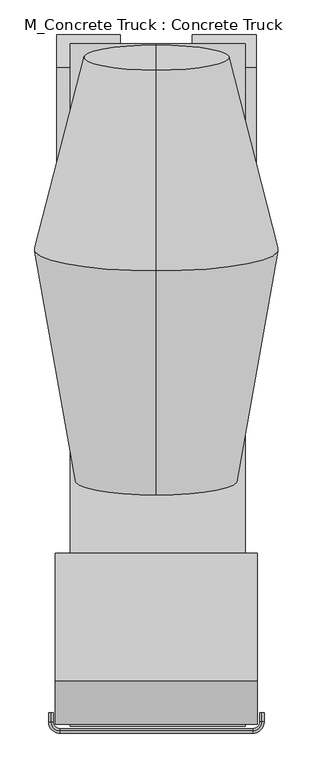
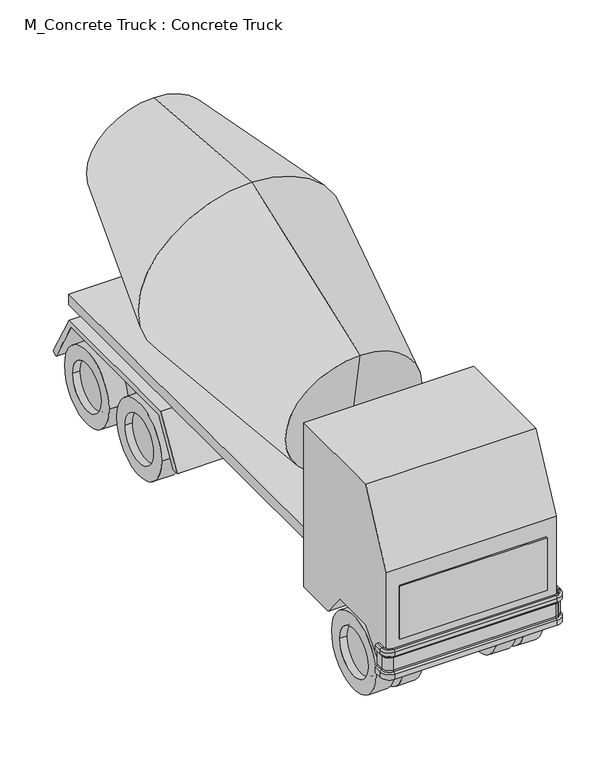
"""IFC4 building model written with IfcOpenShell, lengths in millimetres: geographic element geometry, M_Concrete Truck : Concrete Truck."""

from ifc_helpers import new_model, si_unit, point, frame, frame_2d, origin, place, context, project, spatial, polyline, circle_curve, ellipse_curve, trimmed, segment, composite_curve, outline, extrude, source, transform, mapped, element, save
from ifc_brep_helpers import plane_surface, cylinder_surface, revolved_surface, advanced_brep


def m_concrete_truck_concrete_truck_8dc9909d(model_context):
    return source(origin(), model_context, "Body", "SolidModel", [
        extrude(outline(polyline([(362.4384615, 3777.7615385), (362.4384615, -1683.2384615), (725.7603556, -1683.2384615), (725.7603556, -3004.0384615), (-798.2396444, -3004.0384615), (-798.2396444, -1683.2384615), (-450.3615385, -1683.2384615), (-450.3615385, 3777.7615385), (362.4384615, 3777.7615385)])), frame((0.0, 0.0, 711.2), z_axis=(0.0, 0.0, 1.0), x_axis=(1.0, 0.0, 0.0)), (0.0, 0.0, 1.0), 508.0),
        extrude(outline(composite_curve([segment(trimmed(circle_curve(frame_2d((3091.9615385, 514.35)), 520.7), [point((3612.6615385, 514.35))], [point((2571.2615385, 514.35))], False, "CARTESIAN"), True, "CONTINUOUS"), segment(trimmed(circle_curve(frame_2d((3091.9615385, 514.35)), 520.7), [point((2571.2615385, 514.35))], [point((3612.6615385, 514.35))], False, "CARTESIAN"), True, "CONTINUOUS")], self_intersect=False), holes=[composite_curve([segment(trimmed(circle_curve(frame_2d((3091.9615385, 514.35)), 330.2), [point((3422.1615385, 514.35))], [point((2761.7615385, 514.35))], True, "CARTESIAN"), True, "CONTINUOUS"), segment(trimmed(circle_curve(frame_2d((3091.9615385, 514.35)), 330.2), [point((2761.7615385, 514.35))], [point((3422.1615385, 514.35))], True, "CARTESIAN"), True, "CONTINUOUS")], self_intersect=False)]), frame((829.1634615, 0.0, 0.0), z_axis=(1.0, 0.0, 0.0), x_axis=(0.0, 1.0, 0.0)), (0.0, 0.0, 1.0), 254.0),
        extrude(outline(composite_curve([segment(trimmed(circle_curve(frame_2d((-3131.0384615, 514.35)), 520.7), [point((-2610.3384615, 514.35))], [point((-3651.7384615, 514.35))], False, "CARTESIAN"), True, "CONTINUOUS"), segment(trimmed(circle_curve(frame_2d((-3131.0384615, 514.35)), 520.7), [point((-3651.7384615, 514.35))], [point((-2610.3384615, 514.35))], False, "CARTESIAN"), True, "CONTINUOUS")], self_intersect=False), holes=[composite_curve([segment(trimmed(circle_curve(frame_2d((-3131.0384615, 514.35)), 330.2), [point((-2800.8384615, 514.35))], [point((-3461.2384615, 514.35))], True, "CARTESIAN"), True, "CONTINUOUS"), segment(trimmed(circle_curve(frame_2d((-3131.0384615, 514.35)), 330.2), [point((-3461.2384615, 514.35))], [point((-2800.8384615, 514.35))], True, "CARTESIAN"), True, "CONTINUOUS")], self_intersect=False)]), frame((829.1634615, 0.0, 0.0), z_axis=(1.0, 0.0, 0.0), x_axis=(0.0, 1.0, 0.0)), (0.0, 0.0, 1.0), 254.0),
        extrude(outline(composite_curve([segment(trimmed(circle_curve(frame_2d((1872.7615385, 514.35)), 520.7), [point((2393.4615385, 514.35))], [point((1352.0615385, 514.35))], False, "CARTESIAN"), True, "CONTINUOUS"), segment(trimmed(circle_curve(frame_2d((1872.7615385, 514.35)), 520.7), [point((1352.0615385, 514.35))], [point((2393.4615385, 514.35))], False, "CARTESIAN"), True, "CONTINUOUS")], self_intersect=False), holes=[composite_curve([segment(trimmed(circle_curve(frame_2d((1872.7615385, 514.35)), 330.2), [point((2202.9615385, 514.35))], [point((1542.5615385, 514.35))], True, "CARTESIAN"), True, "CONTINUOUS"), segment(trimmed(circle_curve(frame_2d((1872.7615385, 514.35)), 330.2), [point((1542.5615385, 514.35))], [point((2202.9615385, 514.35))], True, "CARTESIAN"), True, "CONTINUOUS")], self_intersect=False)]), frame((829.1634615, 0.0, 0.0), z_axis=(1.0, 0.0, 0.0), x_axis=(0.0, 1.0, 0.0)), (0.0, 0.0, 1.0), 254.0),
        advanced_brep(
        [(-1212.3615385, -3791.4384615, 661.0144121), (-1263.1615385, -3791.4384615, 661.0144121), (-1263.1615385, -3791.4384615, 734.1328754), (-1243.6602579, -3791.4384615, 753.634156), (-1236.2207701, -3791.4384615, 771.5946682), (-1236.2207701, -3791.4384615, 953.7526192), (-1243.6602579, -3791.4384615, 971.7131315), (-1263.1615385, -3791.4384615, 991.2144121), (-1263.1615385, -3791.4384615, 1042.0144121), (-1237.7615385, -3791.4384615, 1067.4144121), (-1212.3615385, -3791.4384615, 1067.4144121), (-1212.3615385, -3893.0384615, 661.0144121), (-1263.1615385, -3893.0384615, 661.0144121), (-1263.1615385, -3893.0384615, 734.1328754), (-1243.6602579, -3893.0384615, 753.634156), (-1236.2207701, -3893.0384615, 771.5946682), (-1236.2207701, -3893.0384615, 953.7526192), (-1243.6602579, -3893.0384615, 971.7131315), (-1263.1615385, -3893.0384615, 991.2144121), (-1263.1615385, -3893.0384615, 1042.0144121), (-1237.7615385, -3893.0384615, 1067.4144121), (-1212.3615385, -3893.0384615, 1067.4144121), (-1136.1615385, -4020.0384615, 661.0144121), (-1136.1615385, -3969.2384615, 661.0144121), (-1136.1615385, -4020.0384615, 734.1328754), (-1136.1615385, -4000.5371809, 753.634156), (-1136.1615385, -3993.0976932, 771.5946682), (-1136.1615385, -3993.0976932, 953.7526192), (-1136.1615385, -4000.5371809, 971.7131315), (-1136.1615385, -4020.0384615, 991.2144121), (-1136.1615385, -4020.0384615, 1042.0144121), (-1136.1615385, -3994.6384615, 1067.4144121), (-1136.1615385, -3969.2384615, 1067.4144121), (1048.2384615, -3969.2384615, 661.0144121), (1048.2384615, -4020.0384615, 661.0144121), (1048.2384615, -4020.0384615, 734.1328754), (1048.2384615, -4000.5371809, 753.634156), (1048.2384615, -3993.0976932, 771.5946682), (1048.2384615, -3993.0976932, 953.7526192), (1048.2384615, -4000.5371809, 971.7131315), (1048.2384615, -4020.0384615, 991.2144121), (1048.2384615, -4020.0384615, 1042.0144121), (1048.2384615, -3994.6384615, 1067.4144121), (1048.2384615, -3969.2384615, 1067.4144121), (1175.2384615, -3893.0384615, 661.0144121), (1124.4384615, -3893.0384615, 661.0144121), (1175.2384615, -3893.0384615, 734.1328754), (1155.7371809, -3893.0384615, 753.634156), (1148.2976932, -3893.0384615, 771.5946682), (1148.2976932, -3893.0384615, 953.7526192), (1155.7371809, -3893.0384615, 971.7131315), (1175.2384615, -3893.0384615, 991.2144121), (1175.2384615, -3893.0384615, 1042.0144121), (1149.8384615, -3893.0384615, 1067.4144121), (1124.4384615, -3893.0384615, 1067.4144121), (1124.4384615, -3791.4384615, 661.0144121), (1124.4384615, -3791.4384615, 1067.4144121), (1149.8384615, -3791.4384615, 1067.4144121), (1175.2384615, -3791.4384615, 1042.0144121), (1175.2384615, -3791.4384615, 991.2144121), (1155.7371809, -3791.4384615, 971.7131315), (1148.2976932, -3791.4384615, 953.7526192), (1148.2976932, -3791.4384615, 771.5946682), (1155.7371809, -3791.4384615, 753.634156), (1175.2384615, -3791.4384615, 734.1328754), (1175.2384615, -3791.4384615, 661.0144121)],
        [
            (0, 1),
            (1, 2),
            (2, 3),
            (3, 4, circle_curve(frame((-1261.6207701, -3791.4384615, 771.5946682), z_axis=(0.0, -1.0, 0.0), x_axis=(1.0, 0.0, 0.0)), 25.4)),
            (4, 5),
            (5, 6, circle_curve(frame((-1261.6207701, -3791.4384615, 953.7526192), z_axis=(0.0, -1.0, 0.0), x_axis=(1.0, 0.0, 0.0)), 25.4)),
            (6, 7),
            (7, 8),
            (8, 9, circle_curve(frame((-1237.7615385, -3791.4384615, 1042.0144121), z_axis=(0.0, 1.0, 0.0), x_axis=(1.0, 0.0, 0.0)), 25.4)),
            (9, 10),
            (10, 0),
            (0, 11),
            (11, 12),
            (12, 1),
            (12, 13),
            (13, 2),
            (13, 14),
            (14, 3),
            (14, 15, circle_curve(frame((-1261.6207701, -3893.0384615, 771.5946682), z_axis=(0.0, -1.0, 0.0), x_axis=(1.0, 0.0, 0.0)), 25.4)),
            (15, 4),
            (15, 16),
            (16, 5),
            (16, 17, circle_curve(frame((-1261.6207701, -3893.0384615, 953.7526192), z_axis=(0.0, -1.0, 0.0), x_axis=(1.0, 0.0, 0.0)), 25.4)),
            (17, 6),
            (17, 18),
            (18, 7),
            (18, 19),
            (19, 8),
            (19, 20, circle_curve(frame((-1237.7615385, -3893.0384615, 1042.0144121), z_axis=(0.0, 1.0, 0.0), x_axis=(1.0, 0.0, 0.0)), 25.4)),
            (20, 9),
            (20, 21),
            (21, 10),
            (21, 11),
            (22, 12, circle_curve(frame((-1136.1615385, -3893.0384615, 661.0144121), z_axis=(0.0, 0.0, -1.0), x_axis=(-1.0, 0.0, 0.0)), 127.0)),
            (11, 23, circle_curve(frame((-1136.1615385, -3893.0384615, 661.0144121), z_axis=(0.0, 0.0, 1.0), x_axis=(-1.0, 0.0, 0.0)), 76.2)),
            (23, 22),
            (24, 13, circle_curve(frame((-1136.1615385, -3893.0384615, 734.1328754), z_axis=(0.0, 0.0, -1.0), x_axis=(-1.0, 0.0, 0.0)), 127.0)),
            (22, 24),
            (25, 14, circle_curve(frame((-1136.1615385, -3893.0384615, 753.634156), z_axis=(0.0, 0.0, -1.0), x_axis=(-1.0, 0.0, 0.0)), 107.4987194)),
            (24, 25),
            (26, 15, circle_curve(frame((-1136.1615385, -3893.0384615, 771.5946682), z_axis=(0.0, 0.0, -1.0), x_axis=(-1.0, 0.0, 0.0)), 100.0592316)),
            (25, 26, circle_curve(frame((-1136.1615385, -4018.4976932, 771.5946682), z_axis=(1.0, 0.0, 0.0), x_axis=(0.0, 1.0, 0.0)), 25.4)),
            (27, 16, circle_curve(frame((-1136.1615385, -3893.0384615, 953.7526192), z_axis=(0.0, 0.0, -1.0), x_axis=(-1.0, 0.0, 0.0)), 100.0592316)),
            (26, 27),
            (28, 17, circle_curve(frame((-1136.1615385, -3893.0384615, 971.7131315), z_axis=(0.0, 0.0, -1.0), x_axis=(-1.0, 0.0, 0.0)), 107.4987194)),
            (27, 28, circle_curve(frame((-1136.1615385, -4018.4976932, 953.7526192), z_axis=(1.0, 0.0, 0.0), x_axis=(0.0, 1.0, 0.0)), 25.4)),
            (29, 18, circle_curve(frame((-1136.1615385, -3893.0384615, 991.2144121), z_axis=(0.0, 0.0, -1.0), x_axis=(-1.0, 0.0, 0.0)), 127.0)),
            (28, 29),
            (30, 19, circle_curve(frame((-1136.1615385, -3893.0384615, 1042.0144121), z_axis=(0.0, 0.0, -1.0), x_axis=(-1.0, 0.0, 0.0)), 127.0)),
            (29, 30),
            (31, 20, circle_curve(frame((-1136.1615385, -3893.0384615, 1067.4144121), z_axis=(0.0, 0.0, -1.0), x_axis=(-1.0, 0.0, 0.0)), 101.6)),
            (30, 31, circle_curve(frame((-1136.1615385, -3994.6384615, 1042.0144121), z_axis=(-1.0, 0.0, 0.0), x_axis=(0.0, 1.0, 0.0)), 25.4)),
            (32, 21, circle_curve(frame((-1136.1615385, -3893.0384615, 1067.4144121), z_axis=(0.0, 0.0, -1.0), x_axis=(-1.0, 0.0, 0.0)), 76.2)),
            (31, 32),
            (32, 23),
            (23, 33),
            (33, 34),
            (34, 22),
            (34, 35),
            (35, 24),
            (35, 36),
            (36, 25),
            (36, 37, circle_curve(frame((1048.2384615, -4018.4976932, 771.5946682), z_axis=(1.0, 0.0, 0.0), x_axis=(0.0, 1.0, 0.0)), 25.4)),
            (37, 26),
            (37, 38),
            (38, 27),
            (38, 39, circle_curve(frame((1048.2384615, -4018.4976932, 953.7526192), z_axis=(1.0, 0.0, 0.0), x_axis=(0.0, 1.0, 0.0)), 25.4)),
            (39, 28),
            (39, 40),
            (40, 29),
            (40, 41),
            (41, 30),
            (41, 42, circle_curve(frame((1048.2384615, -3994.6384615, 1042.0144121), z_axis=(-1.0, 0.0, 0.0), x_axis=(0.0, 1.0, 0.0)), 25.4)),
            (42, 31),
            (42, 43),
            (43, 32),
            (43, 33),
            (44, 34, circle_curve(frame((1048.2384615, -3893.0384615, 661.0144121), z_axis=(0.0, 0.0, -1.0), x_axis=(0.0, -1.0, 0.0)), 127.0)),
            (33, 45, circle_curve(frame((1048.2384615, -3893.0384615, 661.0144121), z_axis=(0.0, 0.0, 1.0), x_axis=(0.0, -1.0, 0.0)), 76.2)),
            (45, 44),
            (46, 35, circle_curve(frame((1048.2384615, -3893.0384615, 734.1328754), z_axis=(0.0, 0.0, -1.0), x_axis=(0.0, -1.0, 0.0)), 127.0)),
            (44, 46),
            (47, 36, circle_curve(frame((1048.2384615, -3893.0384615, 753.634156), z_axis=(0.0, 0.0, -1.0), x_axis=(0.0, -1.0, 0.0)), 107.4987194)),
            (46, 47),
            (48, 37, circle_curve(frame((1048.2384615, -3893.0384615, 771.5946682), z_axis=(0.0, 0.0, -1.0), x_axis=(0.0, -1.0, 0.0)), 100.0592316)),
            (47, 48, circle_curve(frame((1173.6976932, -3893.0384615, 771.5946682), z_axis=(0.0, 1.0, 0.0), x_axis=(-1.0, 0.0, 0.0)), 25.4)),
            (49, 38, circle_curve(frame((1048.2384615, -3893.0384615, 953.7526192), z_axis=(0.0, 0.0, -1.0), x_axis=(0.0, -1.0, 0.0)), 100.0592316)),
            (48, 49),
            (50, 39, circle_curve(frame((1048.2384615, -3893.0384615, 971.7131315), z_axis=(0.0, 0.0, -1.0), x_axis=(0.0, -1.0, 0.0)), 107.4987194)),
            (49, 50, circle_curve(frame((1173.6976932, -3893.0384615, 953.7526192), z_axis=(0.0, 1.0, 0.0), x_axis=(-1.0, 0.0, 0.0)), 25.4)),
            (51, 40, circle_curve(frame((1048.2384615, -3893.0384615, 991.2144121), z_axis=(0.0, 0.0, -1.0), x_axis=(0.0, -1.0, 0.0)), 127.0)),
            (50, 51),
            (52, 41, circle_curve(frame((1048.2384615, -3893.0384615, 1042.0144121), z_axis=(0.0, 0.0, -1.0), x_axis=(0.0, -1.0, 0.0)), 127.0)),
            (51, 52),
            (53, 42, circle_curve(frame((1048.2384615, -3893.0384615, 1067.4144121), z_axis=(0.0, 0.0, -1.0), x_axis=(0.0, -1.0, 0.0)), 101.6)),
            (52, 53, circle_curve(frame((1149.8384615, -3893.0384615, 1042.0144121), z_axis=(0.0, -1.0, 0.0), x_axis=(-1.0, 0.0, 0.0)), 25.4)),
            (54, 43, circle_curve(frame((1048.2384615, -3893.0384615, 1067.4144121), z_axis=(0.0, 0.0, -1.0), x_axis=(0.0, -1.0, 0.0)), 76.2)),
            (53, 54),
            (54, 45),
            (55, 56),
            (56, 57),
            (57, 58, circle_curve(frame((1149.8384615, -3791.4384615, 1042.0144121), z_axis=(0.0, 1.0, 0.0), x_axis=(-1.0, 0.0, 0.0)), 25.4)),
            (58, 59),
            (59, 60),
            (60, 61, circle_curve(frame((1173.6976932, -3791.4384615, 953.7526192), z_axis=(0.0, -1.0, 0.0), x_axis=(-1.0, 0.0, 0.0)), 25.4)),
            (61, 62),
            (62, 63, circle_curve(frame((1173.6976932, -3791.4384615, 771.5946682), z_axis=(0.0, -1.0, 0.0), x_axis=(-1.0, 0.0, 0.0)), 25.4)),
            (63, 64),
            (64, 65),
            (65, 55),
            (45, 55),
            (65, 44),
            (64, 46),
            (63, 47),
            (62, 48),
            (61, 49),
            (60, 50),
            (59, 51),
            (58, 52),
            (57, 53),
            (56, 54),
        ],
        [
            plane_surface(frame((-2331.7840944, -3791.4384615, 0.0), z_axis=(0.0, 1.0, 0.0), x_axis=(0.0, 0.0, -1.0))),
            plane_surface(frame((-1212.3615385, -3791.4384615, 661.0144121), z_axis=(0.0, 0.0, -1.0), x_axis=(0.0, -1.0, 0.0))),
            plane_surface(frame((-1263.1615385, -3791.4384615, 661.0144121), z_axis=(-1.0, 0.0, 0.0), x_axis=(0.0, -1.0, 0.0))),
            plane_surface(frame((-1263.1615385, -3791.4384615, 734.1328754), z_axis=(-0.7071067811866113, 0.0, 0.7071067811864837), x_axis=(0.0, -1.0, 0.0))),
            revolved_surface(polyline([(-1236.2207701, -3893.0384615, 771.5946682), (-1236.2207701, -3791.4384615, 771.5946682)]), (-1261.6207701, -3791.4384615, 771.5946682), (0.0, -1.0, 0.0)),
            plane_surface(frame((-1236.2207701, -3791.4384615, 771.5946682), z_axis=(-1.0, 0.0, 0.0), x_axis=(0.0, -1.0, 0.0))),
            revolved_surface(polyline([(-1236.2207701, -3893.0384615, 953.7526192), (-1236.2207701, -3791.4384615, 953.7526192)]), (-1261.6207701, -3791.4384615, 953.7526192), (0.0, -1.0, 0.0)),
            plane_surface(frame((-1243.6602579, -3791.4384615, 971.7131315), z_axis=(-0.7071067811866555, 0.0, -0.7071067811864395), x_axis=(0.0, -1.0, 0.0))),
            plane_surface(frame((-1263.1615385, -3791.4384615, 991.2144121), z_axis=(-1.0, 0.0, 0.0), x_axis=(0.0, -1.0, 0.0))),
            cylinder_surface(frame((-1237.7615385, -3791.4384615, 1042.0144121), z_axis=(0.0, 1.0, 0.0), x_axis=(1.0, 0.0, 0.0)), 25.4),
            plane_surface(frame((-1237.7615385, -3791.4384615, 1067.4144121), z_axis=(0.0, 0.0, 1.0), x_axis=(0.0, -1.0, 0.0))),
            plane_surface(frame((-1212.3615385, -3791.4384615, 1067.4144121), z_axis=(1.0, 0.0, 0.0), x_axis=(0.0, -1.0, 0.0))),
            plane_surface(frame((-1136.1615385, -3893.0384615, 661.0144121), z_axis=(0.0, 0.0, -1.0), x_axis=(-1.0, 0.0, 0.0))),
            cylinder_surface(frame((-1136.1615385, -3893.0384615, 0.0), z_axis=(0.0, 0.0, 1.0), x_axis=(-1.0, 0.0, 0.0)), 127.0),
            revolved_surface(polyline([(-1263.1615385, -3893.0384615, 734.1328754), (-1243.6602579, -3893.0384615, 753.634156)]), (-1136.1615385, -3893.0384615, 0.0), (0.0, 0.0, 1.0)),
            revolved_surface(trimmed(ellipse_curve(frame((-1261.6207701, -3893.0384615, 771.5946682), z_axis=(0.0, -1.0, 0.0), x_axis=(1.0, 0.0, 0.0)), 25.4, 25.4), [point((-1243.6602579, -3893.0384615, 753.634156))], [point((-1236.2207701, -3893.0384615, 771.5946682))], True, "CARTESIAN"), (-1136.1615385, -3893.0384615, 0.0), (0.0, 0.0, 1.0)),
            cylinder_surface(frame((-1136.1615385, -3893.0384615, 0.0), z_axis=(0.0, 0.0, 1.0), x_axis=(-1.0, 0.0, 0.0)), 100.0592316),
            revolved_surface(trimmed(ellipse_curve(frame((-1261.6207701, -3893.0384615, 953.7526192), z_axis=(0.0, -1.0, 0.0), x_axis=(1.0, 0.0, 0.0)), 25.4, 25.4), [point((-1236.2207701, -3893.0384615, 953.7526192))], [point((-1243.6602579, -3893.0384615, 971.7131315))], True, "CARTESIAN"), (-1136.1615385, -3893.0384615, 0.0), (0.0, 0.0, 1.0)),
            revolved_surface(polyline([(-1243.6602579, -3893.0384615, 971.7131315), (-1263.1615385, -3893.0384615, 991.2144121)]), (-1136.1615385, -3893.0384615, 0.0), (0.0, 0.0, 1.0)),
            revolved_surface(trimmed(ellipse_curve(frame((-1237.7615385, -3893.0384615, 1042.0144121), z_axis=(0.0, 1.0, 0.0), x_axis=(1.0, 0.0, 0.0)), 25.4, 25.4), [point((-1263.1615385, -3893.0384615, 1042.0144121))], [point((-1237.7615385, -3893.0384615, 1067.4144121))], True, "CARTESIAN"), (-1136.1615385, -3893.0384615, 0.0), (0.0, 0.0, 1.0)),
            plane_surface(frame((-1136.1615385, -3893.0384615, 1067.4144121), z_axis=(0.0, 0.0, 1.0), x_axis=(-1.0, 0.0, 0.0))),
            revolved_surface(polyline([(-1212.3615385, -3893.0384615, 1067.4144121), (-1212.3615385, -3893.0384615, 661.0144121)]), (-1136.1615385, -3893.0384615, 0.0), (0.0, 0.0, 1.0)),
            plane_surface(frame((-1136.1615385, -3969.2384615, 661.0144121), z_axis=(0.0, 0.0, -1.0), x_axis=(1.0, 0.0, 0.0))),
            plane_surface(frame((-1136.1615385, -4020.0384615, 661.0144121), z_axis=(0.0, -1.0, 0.0), x_axis=(1.0, 0.0, 0.0))),
            plane_surface(frame((-1136.1615385, -4020.0384615, 734.1328754), z_axis=(0.0, -0.7071067811866113, 0.7071067811864837), x_axis=(1.0, 0.0, 0.0))),
            revolved_surface(polyline([(1048.2384615, -3993.0976932, 771.5946682), (-1136.1615385, -3993.0976932, 771.5946682)]), (-1136.1615385, -4018.4976932, 771.5946682), (1.0, 0.0, 0.0)),
            plane_surface(frame((-1136.1615385, -3993.0976932, 771.5946682), z_axis=(0.0, -1.0, 0.0), x_axis=(1.0, 0.0, 0.0))),
            revolved_surface(polyline([(1048.2384615, -3993.0976932, 953.7526192), (-1136.1615385, -3993.0976932, 953.7526192)]), (-1136.1615385, -4018.4976932, 953.7526192), (1.0, 0.0, 0.0)),
            plane_surface(frame((-1136.1615385, -4000.5371809, 971.7131315), z_axis=(0.0, -0.7071067811866555, -0.7071067811864395), x_axis=(1.0, 0.0, 0.0))),
            plane_surface(frame((-1136.1615385, -4020.0384615, 991.2144121), z_axis=(0.0, -1.0, 0.0), x_axis=(1.0, 0.0, 0.0))),
            cylinder_surface(frame((-1136.1615385, -3994.6384615, 1042.0144121), z_axis=(-1.0, 0.0, 0.0), x_axis=(0.0, 1.0, 0.0)), 25.4),
            plane_surface(frame((-1136.1615385, -3994.6384615, 1067.4144121), z_axis=(0.0, 0.0, 1.0), x_axis=(1.0, 0.0, 0.0))),
            plane_surface(frame((-1136.1615385, -3969.2384615, 1067.4144121), z_axis=(0.0, 1.0, 0.0), x_axis=(1.0, 0.0, 0.0))),
            plane_surface(frame((1048.2384615, -3893.0384615, 661.0144121), z_axis=(0.0, 0.0, -1.0), x_axis=(0.0, -1.0, 0.0))),
            cylinder_surface(frame((1048.2384615, -3893.0384615, 0.0), z_axis=(0.0, 0.0, 1.0), x_axis=(0.0, -1.0, 0.0)), 127.0),
            revolved_surface(polyline([(1048.2384615, -4020.0384615, 734.1328754), (1048.2384615, -4000.5371809, 753.634156)]), (1048.2384615, -3893.0384615, 0.0), (0.0, 0.0, 1.0)),
            revolved_surface(trimmed(ellipse_curve(frame((1048.2384615, -4018.4976932, 771.5946682), z_axis=(1.0, 0.0, 0.0), x_axis=(0.0, 1.0, 0.0)), 25.4, 25.4), [point((1048.2384615, -4000.5371809, 753.634156))], [point((1048.2384615, -3993.0976932, 771.5946682))], True, "CARTESIAN"), (1048.2384615, -3893.0384615, 0.0), (0.0, 0.0, 1.0)),
            cylinder_surface(frame((1048.2384615, -3893.0384615, 0.0), z_axis=(0.0, 0.0, 1.0), x_axis=(0.0, -1.0, 0.0)), 100.0592316),
            revolved_surface(trimmed(ellipse_curve(frame((1048.2384615, -4018.4976932, 953.7526192), z_axis=(1.0, 0.0, 0.0), x_axis=(0.0, 1.0, 0.0)), 25.4, 25.4), [point((1048.2384615, -3993.0976932, 953.7526192))], [point((1048.2384615, -4000.5371809, 971.7131315))], True, "CARTESIAN"), (1048.2384615, -3893.0384615, 0.0), (0.0, 0.0, 1.0)),
            revolved_surface(polyline([(1048.2384615, -4000.5371809, 971.7131315), (1048.2384615, -4020.0384615, 991.2144121)]), (1048.2384615, -3893.0384615, 0.0), (0.0, 0.0, 1.0)),
            revolved_surface(trimmed(ellipse_curve(frame((1048.2384615, -3994.6384615, 1042.0144121), z_axis=(-1.0, 0.0, 0.0), x_axis=(0.0, 1.0, 0.0)), 25.4, 25.4), [point((1048.2384615, -4020.0384615, 1042.0144121))], [point((1048.2384615, -3994.6384615, 1067.4144121))], True, "CARTESIAN"), (1048.2384615, -3893.0384615, 0.0), (0.0, 0.0, 1.0)),
            plane_surface(frame((1048.2384615, -3893.0384615, 1067.4144121), z_axis=(0.0, 0.0, 1.0), x_axis=(0.0, -1.0, 0.0))),
            revolved_surface(polyline([(1048.2384615, -3969.2384614999996, 1067.4144121), (1048.2384615, -3969.2384614999996, 661.0144121)]), (1048.2384615, -3893.0384615, 0.0), (0.0, 0.0, 1.0)),
            plane_surface(frame((106.6159056, -3791.4384615, 0.0), z_axis=(0.0, 1.0, 0.0), x_axis=(0.0, 0.0, 1.0))),
            plane_surface(frame((1124.4384615, -3893.0384615, 661.0144121), z_axis=(0.0, 0.0, -1.0), x_axis=(0.0, 1.0, 0.0))),
            plane_surface(frame((1175.2384615, -3893.0384615, 661.0144121), z_axis=(1.0, 0.0, 0.0), x_axis=(0.0, 1.0, 0.0))),
            plane_surface(frame((1175.2384615, -3893.0384615, 734.1328754), z_axis=(0.7071067811866113, 0.0, 0.7071067811864837), x_axis=(0.0, 1.0, 0.0))),
            revolved_surface(polyline([(1148.2976932, -3791.4384615, 771.5946682), (1148.2976932, -3893.0384615, 771.5946682)]), (1173.6976932, -3893.0384615, 771.5946682), (0.0, 1.0, 0.0)),
            plane_surface(frame((1148.2976932, -3893.0384615, 771.5946682), z_axis=(1.0, 0.0, 0.0), x_axis=(0.0, 1.0, 0.0))),
            revolved_surface(polyline([(1148.2976932, -3791.4384615, 953.7526192), (1148.2976932, -3893.0384615, 953.7526192)]), (1173.6976932, -3893.0384615, 953.7526192), (0.0, 1.0, 0.0)),
            plane_surface(frame((1155.7371809, -3893.0384615, 971.7131315), z_axis=(0.7071067811866555, 0.0, -0.7071067811864395), x_axis=(0.0, 1.0, 0.0))),
            plane_surface(frame((1175.2384615, -3893.0384615, 991.2144121), z_axis=(1.0, 0.0, 0.0), x_axis=(0.0, 1.0, 0.0))),
            cylinder_surface(frame((1149.8384615, -3893.0384615, 1042.0144121), z_axis=(0.0, -1.0, 0.0), x_axis=(-1.0, 0.0, 0.0)), 25.4),
            plane_surface(frame((1149.8384615, -3893.0384615, 1067.4144121), z_axis=(0.0, 0.0, 1.0), x_axis=(0.0, 1.0, 0.0))),
            plane_surface(frame((1124.4384615, -3893.0384615, 1067.4144121), z_axis=(-1.0, 0.0, 0.0), x_axis=(0.0, 1.0, 0.0))),
        ],
        [
            (0, [[1, 2, 3, 4, 5, 6, 7, 8, 9, 10, 11]]),
            (1, [[-1, 12, 13, 14]]),
            (2, [[-2, -14, 15, 16]]),
            (3, [[-3, -16, 17, 18]]),
            (4, [[-4, -18, 19, 20]]),
            (5, [[-5, -20, 21, 22]]),
            (6, [[-6, -22, 23, 24]]),
            (7, [[-7, -24, 25, 26]]),
            (8, [[-8, -26, 27, 28]]),
            (9, [[-9, -28, 29, 30]]),
            (10, [[-10, -30, 31, 32]]),
            (11, [[-11, -32, 33, -12]]),
            (12, [[34, -13, 35, 36]]),
            (13, [[37, -15, -34, 38]]),
            (14, [[39, -17, -37, 40]]),
            (15, [[41, -19, -39, 42]]),
            (16, [[43, -21, -41, 44]]),
            (17, [[45, -23, -43, 46]]),
            (18, [[47, -25, -45, 48]]),
            (13, [[49, -27, -47, 50]]),
            (19, [[51, -29, -49, 52]]),
            (20, [[53, -31, -51, 54]]),
            (21, [[-35, -33, -53, 55]]),
            (22, [[-36, 56, 57, 58]]),
            (23, [[-38, -58, 59, 60]]),
            (24, [[-40, -60, 61, 62]]),
            (25, [[-42, -62, 63, 64]]),
            (26, [[-44, -64, 65, 66]]),
            (27, [[-46, -66, 67, 68]]),
            (28, [[-48, -68, 69, 70]]),
            (29, [[-50, -70, 71, 72]]),
            (30, [[-52, -72, 73, 74]]),
            (31, [[-54, -74, 75, 76]]),
            (32, [[-55, -76, 77, -56]]),
            (33, [[78, -57, 79, 80]]),
            (34, [[81, -59, -78, 82]]),
            (35, [[83, -61, -81, 84]]),
            (36, [[85, -63, -83, 86]]),
            (37, [[87, -65, -85, 88]]),
            (38, [[89, -67, -87, 90]]),
            (39, [[91, -69, -89, 92]]),
            (34, [[93, -71, -91, 94]]),
            (40, [[95, -73, -93, 96]]),
            (41, [[97, -75, -95, 98]]),
            (42, [[-79, -77, -97, 99]]),
            (43, [[100, 101, 102, 103, 104, 105, 106, 107, 108, 109, 110]]),
            (44, [[-80, 111, -110, 112]]),
            (45, [[-82, -112, -109, 113]]),
            (46, [[-84, -113, -108, 114]]),
            (47, [[-86, -114, -107, 115]]),
            (48, [[-88, -115, -106, 116]]),
            (49, [[-90, -116, -105, 117]]),
            (50, [[-92, -117, -104, 118]]),
            (51, [[-94, -118, -103, 119]]),
            (52, [[-96, -119, -102, 120]]),
            (53, [[-98, -120, -101, 121]]),
            (54, [[-99, -121, -100, -111]]),
        ],
    ),
        extrude(outline(composite_curve([segment(trimmed(circle_curve(frame_2d((3091.9615385, 514.35)), 520.7), [point((3612.6615385, 514.35))], [point((2571.2615385, 514.35))], False, "CARTESIAN"), True, "CONTINUOUS"), segment(trimmed(circle_curve(frame_2d((3091.9615385, 514.35)), 520.7), [point((2571.2615385, 514.35))], [point((3612.6615385, 514.35))], False, "CARTESIAN"), True, "CONTINUOUS")], self_intersect=False), holes=[composite_curve([segment(trimmed(circle_curve(frame_2d((3091.9615385, 514.35)), 330.2), [point((3422.1615385, 514.35))], [point((2761.7615385, 514.35))], True, "CARTESIAN"), True, "CONTINUOUS"), segment(trimmed(circle_curve(frame_2d((3091.9615385, 514.35)), 330.2), [point((2761.7615385, 514.35))], [point((3422.1615385, 514.35))], True, "CARTESIAN"), True, "CONTINUOUS")], self_intersect=False)]), frame((-1171.0865385, 0.0, 0.0), z_axis=(1.0, 0.0, 0.0), x_axis=(0.0, 1.0, 0.0)), (0.0, 0.0, 1.0), 254.0),
        extrude(outline(composite_curve([segment(trimmed(circle_curve(frame_2d((-3131.0384615, 514.35)), 520.7), [point((-2610.3384615, 514.35))], [point((-3651.7384615, 514.35))], False, "CARTESIAN"), True, "CONTINUOUS"), segment(trimmed(circle_curve(frame_2d((-3131.0384615, 514.35)), 520.7), [point((-3651.7384615, 514.35))], [point((-2610.3384615, 514.35))], False, "CARTESIAN"), True, "CONTINUOUS")], self_intersect=False), holes=[composite_curve([segment(trimmed(circle_curve(frame_2d((-3131.0384615, 514.35)), 330.2), [point((-2800.8384615, 514.35))], [point((-3461.2384615, 514.35))], True, "CARTESIAN"), True, "CONTINUOUS"), segment(trimmed(circle_curve(frame_2d((-3131.0384615, 514.35)), 330.2), [point((-3461.2384615, 514.35))], [point((-2800.8384615, 514.35))], True, "CARTESIAN"), True, "CONTINUOUS")], self_intersect=False)]), frame((-1171.0865385, 0.0, 0.0), z_axis=(1.0, 0.0, 0.0), x_axis=(0.0, 1.0, 0.0)), (0.0, 0.0, 1.0), 254.0),
        extrude(outline(composite_curve([segment(trimmed(circle_curve(frame_2d((1872.7615385, 514.35)), 520.7), [point((2393.4615385, 514.35))], [point((1352.0615385, 514.35))], False, "CARTESIAN"), True, "CONTINUOUS"), segment(trimmed(circle_curve(frame_2d((1872.7615385, 514.35)), 520.7), [point((1352.0615385, 514.35))], [point((2393.4615385, 514.35))], False, "CARTESIAN"), True, "CONTINUOUS")], self_intersect=False), holes=[composite_curve([segment(trimmed(circle_curve(frame_2d((1872.7615385, 514.35)), 330.2), [point((2202.9615385, 514.35))], [point((1542.5615385, 514.35))], True, "CARTESIAN"), True, "CONTINUOUS"), segment(trimmed(circle_curve(frame_2d((1872.7615385, 514.35)), 330.2), [point((1542.5615385, 514.35))], [point((2202.9615385, 514.35))], True, "CARTESIAN"), True, "CONTINUOUS")], self_intersect=False)]), frame((-1171.0865385, 0.0, 0.0), z_axis=(1.0, 0.0, 0.0), x_axis=(0.0, 1.0, 0.0)), (0.0, 0.0, 1.0), 254.0),
        extrude(outline(composite_curve([segment(trimmed(circle_curve(frame_2d((3091.9615385, 514.35)), 520.7), [point((3612.6615385, 514.35))], [point((2571.2615385, 514.35))], False, "CARTESIAN"), True, "CONTINUOUS"), segment(trimmed(circle_curve(frame_2d((3091.9615385, 514.35)), 520.7), [point((2571.2615385, 514.35))], [point((3612.6615385, 514.35))], False, "CARTESIAN"), True, "CONTINUOUS")], self_intersect=False)), frame((464.0384615, 0.0, 0.0), z_axis=(1.0, 0.0, 0.0), x_axis=(0.0, 1.0, 0.0)), (0.0, 0.0, 1.0), 254.0),
        extrude(outline(composite_curve([segment(trimmed(circle_curve(frame_2d((-3131.0384615, 514.35)), 520.7), [point((-2610.3384615, 514.35))], [point((-3651.7384615, 514.35))], False, "CARTESIAN"), True, "CONTINUOUS"), segment(trimmed(circle_curve(frame_2d((-3131.0384615, 514.35)), 520.7), [point((-3651.7384615, 514.35))], [point((-2610.3384615, 514.35))], False, "CARTESIAN"), True, "CONTINUOUS")], self_intersect=False)), frame((464.0384615, 0.0, 0.0), z_axis=(1.0, 0.0, 0.0), x_axis=(0.0, 1.0, 0.0)), (0.0, 0.0, 1.0), 254.0),
        extrude(outline(composite_curve([segment(trimmed(circle_curve(frame_2d((1872.7615385, 514.35)), 520.7), [point((2393.4615385, 514.35))], [point((1352.0615385, 514.35))], False, "CARTESIAN"), True, "CONTINUOUS"), segment(trimmed(circle_curve(frame_2d((1872.7615385, 514.35)), 520.7), [point((1352.0615385, 514.35))], [point((2393.4615385, 514.35))], False, "CARTESIAN"), True, "CONTINUOUS")], self_intersect=False)), frame((464.0384615, 0.0, 0.0), z_axis=(1.0, 0.0, 0.0), x_axis=(0.0, 1.0, 0.0)), (0.0, 0.0, 1.0), 254.0),
        extrude(outline(composite_curve([segment(trimmed(circle_curve(frame_2d((3091.9615385, 514.35)), 520.7), [point((3612.6615385, 514.35))], [point((2571.2615385, 514.35))], False, "CARTESIAN"), True, "CONTINUOUS"), segment(trimmed(circle_curve(frame_2d((3091.9615385, 514.35)), 520.7), [point((2571.2615385, 514.35))], [point((3612.6615385, 514.35))], False, "CARTESIAN"), True, "CONTINUOUS")], self_intersect=False)), frame((-805.9615385, 0.0, 0.0), z_axis=(1.0, 0.0, 0.0), x_axis=(0.0, 1.0, 0.0)), (0.0, 0.0, 1.0), 254.0),
        extrude(outline(composite_curve([segment(trimmed(circle_curve(frame_2d((-3139.2915601, 511.4267776)), 520.7), [point((-2618.5915601, 511.4267776))], [point((-3659.9915601, 511.4267776))], False, "CARTESIAN"), True, "CONTINUOUS"), segment(trimmed(circle_curve(frame_2d((-3139.2915601, 511.4267776)), 520.7), [point((-3659.9915601, 511.4267776))], [point((-2618.5915601, 511.4267776))], False, "CARTESIAN"), True, "CONTINUOUS")], self_intersect=False)), frame((-805.9615385, 0.0, 0.0), z_axis=(1.0, 0.0, 0.0), x_axis=(0.0, 1.0, 0.0)), (0.0, 0.0, 1.0), 254.0),
        extrude(outline(composite_curve([segment(trimmed(circle_curve(frame_2d((1872.7615385, 514.35)), 520.7), [point((2393.4615385, 514.35))], [point((1352.0615385, 514.35))], False, "CARTESIAN"), True, "CONTINUOUS"), segment(trimmed(circle_curve(frame_2d((1872.7615385, 514.35)), 520.7), [point((1352.0615385, 514.35))], [point((2393.4615385, 514.35))], False, "CARTESIAN"), True, "CONTINUOUS")], self_intersect=False)), frame((-805.9615385, 0.0, 0.0), z_axis=(1.0, 0.0, 0.0), x_axis=(0.0, 1.0, 0.0)), (0.0, 0.0, 1.0), 254.0),
        extrude(outline(composite_curve([segment(trimmed(circle_curve(frame_2d((-3131.0384615, 514.35)), 330.2), [point((-2800.8384615, 514.35))], [point((-3461.2384615, 514.35))], False, "CARTESIAN"), True, "CONTINUOUS"), segment(trimmed(circle_curve(frame_2d((-3131.0384615, 514.35)), 330.2), [point((-3461.2384615, 514.35))], [point((-2800.8384615, 514.35))], False, "CARTESIAN"), True, "CONTINUOUS")], self_intersect=False)), frame((-1072.859976, 0.0, 0.0), z_axis=(1.0, 0.0, 0.0), x_axis=(0.0, 1.0, 0.0)), (0.0, 0.0, 1.0), 155.7734375),
        extrude(outline(composite_curve([segment(trimmed(circle_curve(frame_2d((1872.7615385, 514.35)), 330.2), [point((2202.9615385, 514.35))], [point((1542.5615385, 514.35))], False, "CARTESIAN"), True, "CONTINUOUS"), segment(trimmed(circle_curve(frame_2d((1872.7615385, 514.35)), 330.2), [point((1542.5615385, 514.35))], [point((2202.9615385, 514.35))], False, "CARTESIAN"), True, "CONTINUOUS")], self_intersect=False)), frame((-1072.859976, 0.0, 0.0), z_axis=(1.0, 0.0, 0.0), x_axis=(0.0, 1.0, 0.0)), (0.0, 0.0, 1.0), 155.7734375),
        extrude(outline(composite_curve([segment(trimmed(circle_curve(frame_2d((3091.9615385, 514.35)), 330.2), [point((3422.1615385, 514.35))], [point((2761.7615385, 514.35))], False, "CARTESIAN"), True, "CONTINUOUS"), segment(trimmed(circle_curve(frame_2d((3091.9615385, 514.35)), 330.2), [point((2761.7615385, 514.35))], [point((3422.1615385, 514.35))], False, "CARTESIAN"), True, "CONTINUOUS")], self_intersect=False)), frame((-1072.859976, 0.0, 0.0), z_axis=(1.0, 0.0, 0.0), x_axis=(0.0, 1.0, 0.0)), (0.0, 0.0, 1.0), 155.7734375),
        extrude(outline(composite_curve([segment(trimmed(circle_curve(frame_2d((-3129.2190592, 514.3449875)), 330.2), [point((-2799.0190592, 514.3449875))], [point((-3459.4190592, 514.3449875))], False, "CARTESIAN"), True, "CONTINUOUS"), segment(trimmed(circle_curve(frame_2d((-3129.2190592, 514.3449875)), 330.2), [point((-3459.4190592, 514.3449875))], [point((-2799.0190592, 514.3449875))], False, "CARTESIAN"), True, "CONTINUOUS")], self_intersect=False)), frame((829.1634615, 0.0, 0.0), z_axis=(1.0, 0.0, 0.0), x_axis=(0.0, 1.0, 0.0)), (0.0, 0.0, 1.0), 172.4421875),
        extrude(outline(composite_curve([segment(trimmed(circle_curve(frame_2d((1874.5809408, 514.3449875)), 330.2), [point((2204.7809408, 514.3449875))], [point((1544.3809408, 514.3449875))], False, "CARTESIAN"), True, "CONTINUOUS"), segment(trimmed(circle_curve(frame_2d((1874.5809408, 514.3449875)), 330.2), [point((1544.3809408, 514.3449875))], [point((2204.7809408, 514.3449875))], False, "CARTESIAN"), True, "CONTINUOUS")], self_intersect=False)), frame((829.1634615, 0.0, 0.0), z_axis=(1.0, 0.0, 0.0), x_axis=(0.0, 1.0, 0.0)), (0.0, 0.0, 1.0), 172.4421875),
        extrude(outline(composite_curve([segment(trimmed(circle_curve(frame_2d((3091.9615385, 514.35)), 330.2), [point((3422.1615385, 514.35))], [point((2761.7615385, 514.35))], False, "CARTESIAN"), True, "CONTINUOUS"), segment(trimmed(circle_curve(frame_2d((3091.9615385, 514.35)), 330.2), [point((2761.7615385, 514.35))], [point((3422.1615385, 514.35))], False, "CARTESIAN"), True, "CONTINUOUS")], self_intersect=False)), frame((829.1634615, 0.0, 0.0), z_axis=(1.0, 0.0, 0.0), x_axis=(0.0, 1.0, 0.0)), (0.0, 0.0, 1.0), 172.4421875),
        extrude(outline(polyline([(-1988.0384615, 3098.8), (-1988.0384615, 762.0), (-2559.5384615, 762.0), (-2843.3895639, 1100.280571), (-3438.6103421, 1100.280571), (-3723.9042167, 760.280571), (-3918.0646084, 760.280571), (-3918.0646084, 2133.6), (-3436.7074529, 3098.8), (-1988.0384615, 3098.8)])), frame((-1186.9615385, 0.0, 0.0), z_axis=(1.0, 0.0, 0.0), x_axis=(0.0, 1.0, 0.0)), (0.0, 0.0, 1.0), 2286.0),
        advanced_brep(
        [(-43.9615385, -1168.0113462, 2355.2104547), (-43.9615385, -1009.570534, 1454.7367752), (-43.9615385, -1326.4521585, 3255.6841343), (-43.9615385, 1686.1636133, 1454.7367752), (-43.9615385, 1207.3779879, 4175.8403069), (-43.9615385, 3762.828493, 2387.7409698), (-43.9615385, 3477.789427, 4007.7161067), (-43.9615385, 3620.30896, 3197.7285383)],
        [
            (0, 1),
            (1, 2, circle_curve(frame((-43.9615385, -1168.0113462, 2355.2104547), z_axis=(0.0, -0.9848707186111331, -0.17329070264267052), x_axis=(0.0, 0.17329070264267052, -0.9848707186111331)), 914.3064795)),
            (2, 0),
            (2, 1, circle_curve(frame((-43.9615385, -1168.0113462, 2355.2104547), z_axis=(0.0, -0.9848707186111331, -0.17329070264267052), x_axis=(0.0, 0.17329070264267052, -0.9848707186111331)), 914.3064795)),
            (1, 3),
            (3, 4, circle_curve(frame((-43.9615385, 1446.7708006, 2815.2885411), z_axis=(0.0, -0.9848707186111331, -0.17329070264267052), x_axis=(0.0, 0.17329070264267052, -0.9848707186111331)), 1381.452144)),
            (4, 2),
            (4, 3, circle_curve(frame((-43.9615385, 1446.7708006, 2815.2885411), z_axis=(0.0, -0.9848707186111331, -0.17329070264267052), x_axis=(0.0, 0.17329070264267052, -0.9848707186111331)), 1381.452144)),
            (3, 5),
            (5, 6, circle_curve(frame((-43.9615385, 3620.30896, 3197.7285383), z_axis=(0.0, -0.9848707186111331, -0.17329070264267052), x_axis=(0.0, 0.17329070264267052, -0.9848707186111331)), 822.4303486)),
            (6, 4),
            (5, 7),
            (7, 6),
            (5, 6, circle_curve(frame((-43.9615385, 3620.30896, 3197.7285383), z_axis=(0.0, 0.9848707186111331, 0.17329070264267052), x_axis=(0.0, 0.17329070264267052, -0.9848707186111331)), 822.4303486)),
        ],
        [
            plane_surface(frame((-43.9615385, -1168.0113462, 2355.2104547), z_axis=(0.0, -0.9848707186111331, -0.17329070264267052), x_axis=(0.0, 0.17329070264267052, -0.9848707186111331))),
            revolved_surface(polyline([(-43.9615385, 1686.1636133, 1454.7367752), (-43.9615385, -1009.570534, 1454.7367752)]), (-43.9615385, -1168.0113462, 2355.2104547), (0.0, -0.9848707186111331, -0.17329070264267052)),
            revolved_surface(polyline([(-43.9615385, 3762.828493, 2387.7409698), (-43.9615385, 1686.1636133, 1454.7367752)]), (-43.9615385, -1168.0113462, 2355.2104547), (0.0, -0.9848707186111331, -0.17329070264267052)),
            plane_surface(frame((-43.9615385, 3620.30896, 3197.7285383), z_axis=(0.0, 0.9848707186111331, 0.17329070264267052), x_axis=(0.0, 0.17329070264267052, -0.9848707186111331))),
        ],
        [
            (0, [[1, 2, 3]]),
            (0, [[-3, 4, -1]]),
            (1, [[-2, 5, 6, 7]]),
            (1, [[-4, -7, 8, -5]]),
            (2, [[-6, 9, 10, 11]]),
            (3, [[-10, 12, 13]]),
            (3, [[14, -13, -12]]),
            (2, [[-8, -11, -14, -9]]),
        ],
    ),
        extrude(outline(polyline([(961.348456, -1988.0384615), (-1019.851544, -1988.0384615), (-1019.851544, 3777.7615385), (961.348456, 3777.7615385), (961.348456, -1988.0384615)])), frame((0.0, 0.0, 1219.2), z_axis=(0.0, 0.0, 1.0), x_axis=(1.0, 0.0, 0.0)), (0.0, 0.0, 1.0), 150.6140625),
        extrude(outline(polyline([(3504.4692149, 1219.2), (3876.2424022, 557.8623027), (3809.818509, 520.5218901), (3459.8903681, 1143.0), (1414.8633054, 1143.0), (1077.8573959, 559.2886423), (989.8692149, 559.2886423), (1370.8692149, 1219.2), (3504.4692149, 1219.2)])), frame((-1171.0865385, 0.0, 0.0), z_axis=(1.0, 0.0, 0.0), x_axis=(0.0, 1.0, 0.0)), (0.0, 0.0, 1.0), 720.725),
        extrude(outline(polyline([(3504.4692149, 1219.2), (3876.2424022, 557.8623027), (3809.818509, 520.5218901), (3459.8903681, 1143.0), (1414.8633054, 1143.0), (1077.8573959, 559.2886423), (989.8692149, 559.2886423), (1370.8692149, 1219.2), (3504.4692149, 1219.2)])), frame((362.4384615, 0.0, 0.0), z_axis=(1.0, 0.0, 0.0), x_axis=(0.0, 1.0, 0.0)), (0.0, 0.0, 1.0), 720.725),
        extrude(outline(polyline([(961.348456, -3941.4802334), (-1020.2612622, -3941.4802334), (-1020.2612622, -3918.0646084), (961.348456, -3918.0646084), (961.348456, -3941.4802334)])), frame((0.0, 0.0, 1143.0), z_axis=(0.0, 0.0, 1.0), x_axis=(1.0, 0.0, 0.0)), (0.0, 0.0, 1.0), 750.2675431),
    ])


if __name__ == "__main__":
    model = new_model("IFC4")
    model_context = context("Model", 3, world=origin())
    ifc_project = project(units=[si_unit("LENGTHUNIT", "METRE", prefix="MILLI")], contexts=[model_context])
    site = spatial("IfcSite", under=ifc_project)
    building = spatial("IfcBuilding", under=site)
    placement = place(None, origin())
    m_concrete_truck_concrete_truck_shape = m_concrete_truck_concrete_truck_8dc9909d(model_context)
    element("IfcGeographicElement", 1, ObjectType="M_Concrete Truck : Concrete Truck", at=placement, inside=building, context=model_context, shape_type="MappedRepresentation", body=[
        mapped(m_concrete_truck_concrete_truck_shape, transform((0.0, 0.0, 0.0), x_axis=(1.0, 0.0, 0.0), y_axis=(0.0, 1.0, 0.0), z_axis=(0.0, 0.0, 1.0))),
    ])
    save(model, "model.ifc")

# Revit data of these elements
# Type "M_Concrete Truck : Concrete Truck"
#   Cab Material = Metal, Paint Finish, White, Matte
#   Tire Material = Plastic, Opaque Black
#   Trailer Material = Metal, Paint Finish, White, Matte
# Element 1 (IfcGeographicElement, "M_Concrete Truck : Concrete Truck")
#   Materials on its faces: "Steel, Chrome Plated", "Plastic, Opaque Black", "Steel", "Metal, Paint Finish, White, Matte"
# Materials
#   "Metal, Paint Finish, White, Matte": class "Metal", colour RGB 247 247 239, transparency 0, Description = "Paint finished steel", Cost = 0
#   "Plastic, Opaque Black": class "Plastic", colour RGB 0 0 0, transparency 0.7, Description = "Plastic, generic, opaque black", Cost = 0
#   "Steel, Chrome Plated": class "Metal", colour RGB 17 17 17, transparency 0, Description = "Chromiuim plated steel", Cost = 0
#   "Steel": class "Metal", colour RGB 128 128 128, transparency 0, Description = "Steel, mill finish", Cost = 0
